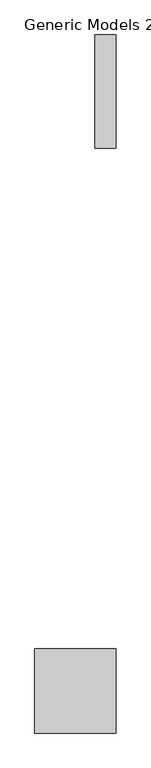
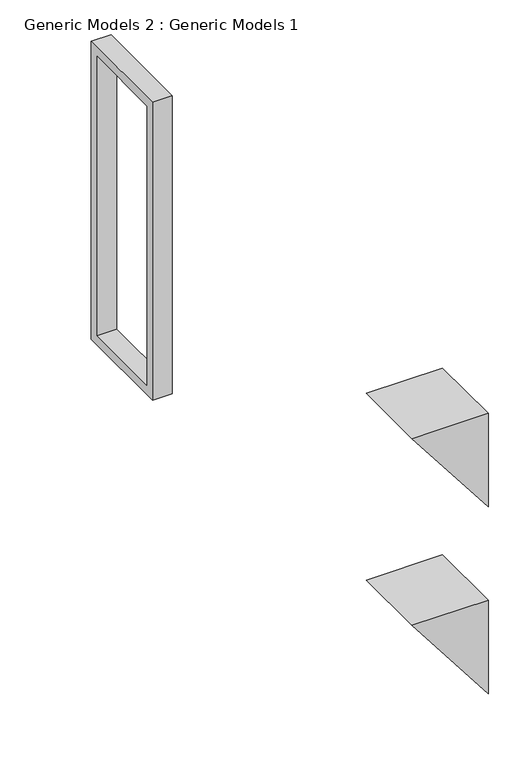
"""IFC4 building model written with IfcOpenShell, lengths in millimetres: proxy geometry, Generic Models 2 : Generic Models 1."""

from ifc_helpers import new_model, si_unit, frame, origin, place, context, project, spatial, polyline, outline, extrude, faceted_brep, source, transform, mapped, element, save


def generic_models_2_generic_models_1_7ae53c19(model_context):
    return source(origin(), model_context, "Body", "SolidModel", [
        faceted_brep([(-15539.3231107, -3758.4534819, 914.4), (-15539.3231107, -3758.4534819, 2438.4), (-15539.3231107, -4977.6534819, 2438.4), (-15539.3231107, -4977.6534819, 914.4), (-15539.3231107, -3910.8534819, 1066.8), (-15539.3231107, -4825.2534819, 1066.8), (-15539.3231107, -4825.2534819, 2286.0), (-15539.3231107, -3910.8534819, 2286.0), (-16596.8434996, -3910.8534819, 2286.0), (-15656.8253761, -3910.8534819, 1066.8), (-16596.8434996, -4825.2534819, 2286.0), (-15656.8253761, -4825.2534819, 1066.8), (-16714.3457651, -4977.6534819, 2438.4), (-16714.3457651, -3758.4534819, 2438.4)], [[[0, 1, 2, 3], [4, 5, 6, 7]], [[4, 7, 8, 9]], [[7, 6, 10, 8]], [[6, 5, 11, 10]], [[5, 4, 9, 11]], [[3, 2, 12]], [[2, 1, 13, 12]], [[1, 0, 13]], [[0, 3, 12, 13], [9, 8, 10, 11]]]),
        faceted_brep([(-15539.3231107, -3758.4534819, 3962.4), (-15539.3231107, -3758.4534819, 5486.4), (-15539.3231107, -4977.6534819, 5486.4), (-15539.3231107, -4977.6534819, 3962.4), (-15539.3231107, -3910.8534819, 4114.8), (-15539.3231107, -4825.2534819, 4114.8), (-15539.3231107, -4825.2534819, 5334.0), (-15539.3231107, -3910.8534819, 5334.0), (-16596.8434996, -3910.8534819, 5334.0), (-15656.8253761, -3910.8534819, 4114.8), (-16596.8434996, -4825.2534819, 5334.0), (-15656.8253761, -4825.2534819, 4114.8), (-16714.3457651, -4977.6534819, 5486.4), (-16714.3457651, -3758.4534819, 5486.4)], [[[0, 1, 2, 3], [4, 5, 6, 7]], [[4, 7, 8, 9]], [[7, 6, 10, 8]], [[6, 5, 11, 10]], [[5, 4, 9, 11]], [[3, 2, 12]], [[2, 1, 13, 12]], [[1, 0, 13]], [[0, 3, 12, 13], [9, 8, 10, 11]]]),
        extrude(outline(polyline([(5112.4965181, 682.6676291), (3474.1965181, 682.6676291), (3474.1965181, 5543.55), (5112.4965181, 5543.55), (5112.4965181, 682.6676291)]), holes=[polyline([(4960.0965181, 835.0676291), (4960.0965181, 5391.15), (3626.5965181, 5391.15), (3626.5965181, 835.0676291), (4960.0965181, 835.0676291)])]), frame((-15844.1231107, 0.0, 0.0), z_axis=(1.0, 0.0, 0.0), x_axis=(0.0, 1.0, 0.0)), (0.0, 0.0, 1.0), 304.8),
    ])


if __name__ == "__main__":
    model = new_model("IFC4")
    model_context = context("Model", 3, world=origin())
    ifc_project = project(units=[si_unit("LENGTHUNIT", "METRE", prefix="MILLI")], contexts=[model_context])
    site = spatial("IfcSite", under=ifc_project)
    building = spatial("IfcBuilding", under=site)
    placement = place(None, origin())
    generic_models_2_generic_models_1_shape = generic_models_2_generic_models_1_7ae53c19(model_context)
    element("IfcBuildingElementProxy", 1, Name="Generic Models 2 : Generic Models 1", ObjectType="Generic Models 2 : Generic Models 1", at=placement, inside=building, context=model_context, shape_type="MappedRepresentation", body=[
        mapped(generic_models_2_generic_models_1_shape, transform((0.0, 0.0, 0.0), x_axis=(1.0, 0.0, 0.0), y_axis=(0.0, 1.0, 0.0), z_axis=(0.0, 0.0, 1.0))),
    ])
    save(model, "model.ifc")
